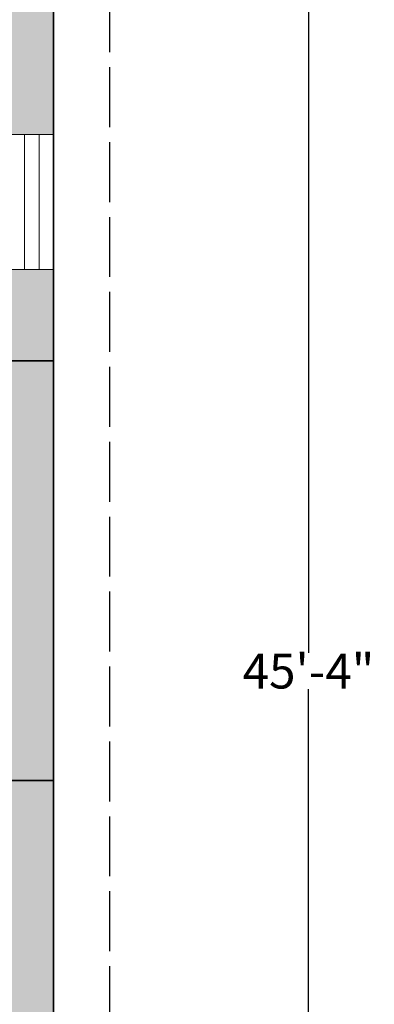
# Model space of a CAD drawing. Units: inches. Extents: x 1316 to 1777, y 813 to 1650.
# Tile 17 of 22: x 1706 to 1777, y 1237 to 1434. Entities that reach past the tile are written whole.
import ezdxf

# ---------------------------------------------------------------- set-up
doc = ezdxf.new("R2010")
doc.units = ezdxf.units.IN
doc.header["$MEASUREMENT"] = 0
doc.linetypes.add('ACAD_ISO02W100', pattern=[15, 12, -3])
for name, color, linetype, lineweight in [('A-ANNO-DIMS', 2, 'Continuous', 18), ('A-WALL-PATT', 250, 'Continuous', 13), ('C-PROP', 8, 'ACAD_ISO02W100', 25), ('walls', 250, 'Continuous', 35), ('windows', 141, 'Continuous', 18)]:
    doc.layers.add(name, color=color, linetype=linetype, lineweight=lineweight)
doc.styles.get("Standard").update_dxf_attribs({"font": 'arial.ttf'})
doc.dimstyles.get("Standard").update_dxf_attribs({"dimtxt": 7, "dimasz": 0.18, "dimexe": 0.18, "dimexo": 0.0625, "dimgap": 0.09, "dimtad": 0, "dimtih": 1, "dimtoh": 1, "dimzin": 0, "dimdsep": 46, "dimlunit": 3, "dimtxsty": 'Standard', "dimcen": 0.09, "dimadec": 0, "dimazin": 0, "dimtfac": 1, "dimtofl": 0, "dimtmove": 0, "dimatfit": 3, "dimfxl": 1, "dimtolj": 1, "dimtzin": 0, "dimarcsym": 0})

# ---------------------------------------------------------------- blocks, each defined once
blk = doc.blocks.new('*D51')
at = {"layer": 'A-ANNO-DIMS', "color": 0, "lineweight": -2, "transparency": 16777216}
for p, q in [((1713.24, 1575.37), (1764.48, 1575.37)), ((1764.3, 1575.19), (1764.3, 1306.92)), ((1764.3, 1031.35), (1764.3, 1299.62)), ((1713.24, 1031.17), (1764.48, 1031.17))]:
    blk.add_line(p, q, dxfattribs=at)
at = {"layer": 'A-ANNO-DIMS', "color": 0, "transparency": 16777216}
for points in [[(1764.27, 1575.19), (1764.33, 1575.19), (1764.3, 1575.37)], [(1764.27, 1031.35), (1764.33, 1031.35), (1764.3, 1031.17)]]:
    blk.add_solid(points, dxfattribs=at)
at = {"layer": 'Defpoints', "color": 0, "transparency": 16777216}
for p in [(1713.17, 1575.37), (1764.3, 1575.37), (1713.17, 1031.17)]:
    blk.add_point(p, dxfattribs=at)
at = {"layer": 'A-ANNO-DIMS', "color": 0, "transparency": 16777216, "insert": (1764.3, 1303.27), "char_height": 7, "attachment_point": 5}
blk.add_mtext('\\A1;45\'-4"', dxfattribs=at)

msp = doc.modelspace()

# ---------------------------------------------------------------- hatches: boundary and pattern name
at = {"layer": 'A-WALL-PATT'}
h = msp.add_hatch(color=256, dxfattribs=at)
h.dxf.hatch_style = 1
h.paths.add_polyline_path([(1713.173, 1281.369), (1656.173, 1281.369), (1656.173, 1298.258), (1651.673, 1298.258), (1651.673, 1281.369), (1567.673, 1281.369), (1567.673, 1266.995), (1572.173, 1266.995), (1572.173, 1276.869), (1704.173, 1276.869), (1704.173, 1132.869), (1608.64, 1132.869), (1608.64, 1123.869), (1704.173, 1123.869), (1704.173, 1040.173), (1652.869, 1040.173), (1652.869, 1031.173), (1713.173, 1031.173), (1713.173, 1040.173)])
h.paths.add_polyline_path([(1572.173, 1237.955), (1567.673, 1237.955), (1567.673, 1123.869), (1583.146, 1123.869), (1583.146, 1132.869), (1572.173, 1132.869)], flags=17)
h.paths.add_polyline_path([(1510.345, 1566.369), (1524.171, 1566.369), (1524.171, 1571.985), (1524.171, 1575.369), (1445.955, 1575.369), (1445.955, 1566.369), (1505.845, 1566.369), (1505.845, 1469.591), (1510.345, 1469.591), (1510.345, 1471.869), (1529.081, 1471.869), (1529.081, 1476.369), (1510.345, 1476.369)])
h.paths.add_polyline_path([(1609.722, 1575.369), (1545.119, 1575.369), (1545.119, 1566.369), (1570.345, 1566.369), (1570.345, 1476.369), (1562.477, 1476.369), (1562.477, 1471.869), (1570.345, 1471.869), (1570.345, 1469.591), (1574.845, 1469.591), (1574.845, 1566.369), (1609.722, 1566.369)])
h.paths.add_polyline_path([(1713.173, 1575.369), (1655.233, 1575.369), (1655.233, 1566.369), (1704.173, 1566.369), (1704.173, 1434.369), (1574.845, 1434.369), (1574.845, 1440.551), (1574.701, 1440.551), (1570.345, 1440.551), (1570.345, 1429.869), (1597.673, 1429.869), (1597.673, 1408.281), (1602.173, 1408.281), (1602.173, 1429.869), (1704.173, 1429.869), (1704.173, 1410.704), (1707.375, 1410.704), (1713.173, 1410.704)])
h.paths.add_polyline_path([(1713.173, 1383.676), (1704.173, 1383.676), (1704.173, 1369.869), (1602.173, 1369.869), (1602.173, 1379.241), (1597.673, 1379.241), (1597.673, 1365.369), (1713.173, 1365.369)])
h.paths.add_polyline_path([(1444.564, 1429.869), (1510.345, 1429.869), (1510.345, 1440.551), (1505.845, 1440.551), (1505.845, 1434.369), (1386.064, 1434.369), (1386.064, 1566.369), (1400.445, 1566.369), (1400.445, 1575.369), (1377.064, 1575.369), (1377.064, 1412.813), (1380.509, 1412.813), (1386.064, 1412.813), (1386.064, 1429.869), (1440.064, 1429.869), (1440.064, 1401.229), (1444.564, 1401.229)])
h.paths.add_polyline_path([(1444.564, 1372.189), (1440.064, 1372.189), (1440.064, 1369.869), (1386.064, 1369.869), (1386.064, 1378.758), (1377.064, 1378.758), (1377.064, 1349.201), (1381.118, 1349.201), (1386.064, 1349.201), (1386.064, 1365.369), (1440.064, 1365.369), (1440.064, 1322.882), (1444.564, 1322.882)])
h.paths.add_polyline_path([(1510.564, 1295.094), (1506.064, 1295.094), (1506.064, 1245.369), (1386.064, 1245.369), (1386.064, 1272.582), (1377.064, 1272.582), (1377.064, 1212.905), (1380.1, 1212.905), (1386.064, 1212.905), (1386.064, 1240.869), (1510.564, 1240.869)])
h.paths.add_polyline_path([(1386.064, 1163.761), (1377.064, 1163.761), (1377.064, 1063.869), (1419.363, 1063.869), (1419.363, 1072.869), (1386.064, 1072.869)])
h.paths.add_polyline_path([(1510.564, 1072.869), (1469.381, 1072.869), (1469.381, 1063.869), (1501.564, 1063.869), (1501.564, 1033.023), (1501.564, 1031.173), (1540.829, 1031.173), (1540.829, 1036.182, -0.0299535), (1541.068, 1040.173), (1510.564, 1040.173)])
h.paths.add_polyline_path([(1607.369, 1040.173), (1574.225, 1040.173), (1574.225, 1036.182), (1574.225, 1031.173), (1607.369, 1031.173)], flags=17)
h.paths.add_polyline_path([(1637.054, 1040.173), (1624.706, 1040.173), (1624.706, 1031.173), (1637.054, 1031.173)], flags=17)
h = msp.add_hatch(color=256, dxfattribs=at)
h.dxf.hatch_style = 1
h.paths.add_polyline_path([(1713.173, 1365.369), (1704.173, 1365.369), (1704.173, 1281.369), (1713.173, 1281.369)])

# ---------------------------------------------------------------- linework, layer by layer
at = {"layer": 'C-PROP'}
msp.add_line((1724.399, 1604.173), (1724.399, 1040.173), dxfattribs=at)
at = {"layer": 'walls'}
for p, q in [((1713.173, 1575.369), (1713.173, 1040.173)), ((1597.673, 1365.369), (1713.173, 1365.369)), ((1656.173, 1281.369), (1713.173, 1281.369))]:
    msp.add_line(p, q, dxfattribs=at)
at = {"layer": 'windows'}
for p, q in [((1704.173, 1410.704), (1713.173, 1410.704)), ((1704.173, 1410.704), (1707.375, 1410.704)), ((1707.375, 1410.704), (1707.375, 1383.676)), ((1710.348, 1383.676), (1710.348, 1410.704)), ((1713.173, 1410.704), (1713.173, 1383.676)), ((1713.173, 1383.676), (1704.173, 1383.676)), ((1707.375, 1383.676), (1710.348, 1383.676))]:
    msp.add_line(p, q, dxfattribs=at)

# ---------------------------------------------------------------- dimensions: what is measured, and where the dimension line sits
at = {"layer": 'A-ANNO-DIMS'}
dim = msp.add_linear_dim(base=(1764.299, 1575.369), p1=(1713.173, 1031.173), p2=(1713.173, 1575.369), angle=90, dimstyle='Standard', override={"dimdec": 1, "dimlfac": 1, "dimrnd": 0, "dimzin": 1, "dimdsep": 46, "dimlunit": 4, "dimfrac": 2}, dxfattribs=at)
dim.commit()
dim.dimension.update_dxf_attribs({"geometry": '*D51', "text_midpoint": (1764.299, 1303.271)})

doc.saveas('drawing.dxf')
